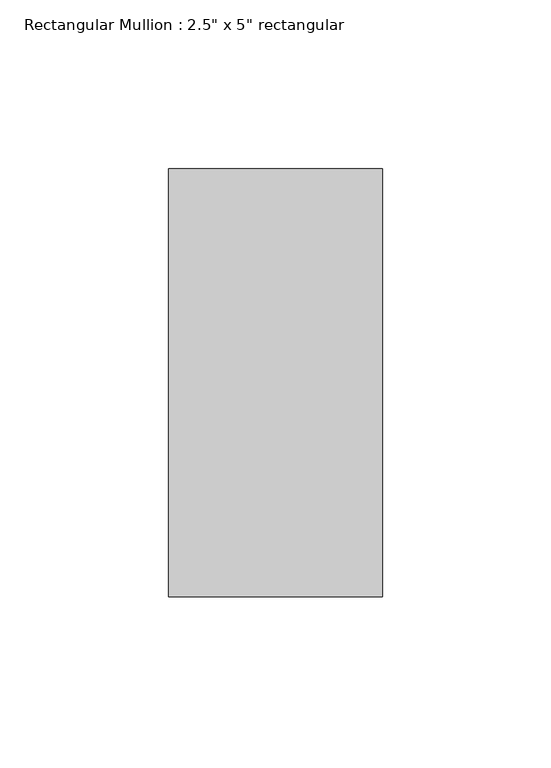
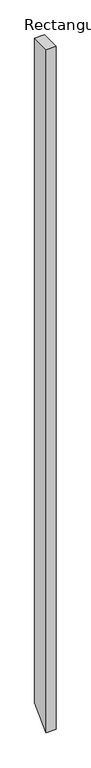
"""IFC4 building model written with IfcOpenShell, lengths in millimetres: member geometry."""

from ifc_helpers import new_model, si_unit, frame, origin, place, context, project, spatial, polyline, outline, extrude, source, transform, mapped, element, save


def member_baaa0d74(model_context):
    return source(origin(), model_context, "Body", "SweptSolid", [
        extrude(outline(polyline([(-63.5, 0.0), (63.5, 0.0), (63.5, -4514.1490316), (-63.5, -4641.1490316), (-63.5, 0.0)])), frame((-63.5, 0.0, 0.0), z_axis=(1.0, 0.0, 0.0), x_axis=(0.0, 1.0, 0.0)), (0.0, 0.0, 1.0), 63.5),
    ])


if __name__ == "__main__":
    model = new_model("IFC4")
    model_context = context("Model", 3, world=origin())
    ifc_project = project(units=[si_unit("LENGTHUNIT", "METRE", prefix="MILLI")], contexts=[model_context])
    site = spatial("IfcSite", under=ifc_project)
    building = spatial("IfcBuilding", under=site)
    placement = place(None, origin())
    member_shape = member_baaa0d74(model_context)
    element("IfcMember", 1, ObjectType="Rectangular Mullion : 2.5\" x 5\" rectangular", at=placement, inside=building, context=model_context, shape_type="MappedRepresentation", body=[
        mapped(member_shape, transform((0.0, 0.0, 0.0), x_axis=(1.0, 0.0, 0.0), y_axis=(0.0, 1.0, 0.0), z_axis=(0.0, 0.0, 1.0))),
    ])
    save(model, "model.ifc")

# Revit data of these elements
# Type "Rectangular Mullion : 2.5\" x 5\" rectangular"
#   built-in parameter 1007304 = 0.416667 (stored number, unit not read)
#   built-in parameter 1007301 = 0.104167 (stored number, unit not read)
#   built-in parameter 1007300 = 0.104167 (stored number, unit not read)
# Element 1 (IfcMember, "Rectangular Mullion : 2.5\" x 5\" rectangular")
#   Materials on its faces: "Aluminum"
# Materials
#   "Aluminum": class "Metal", colour RGB 247 247 247, transparency 0, Description = "Aluminum 6061", Cost = 0
